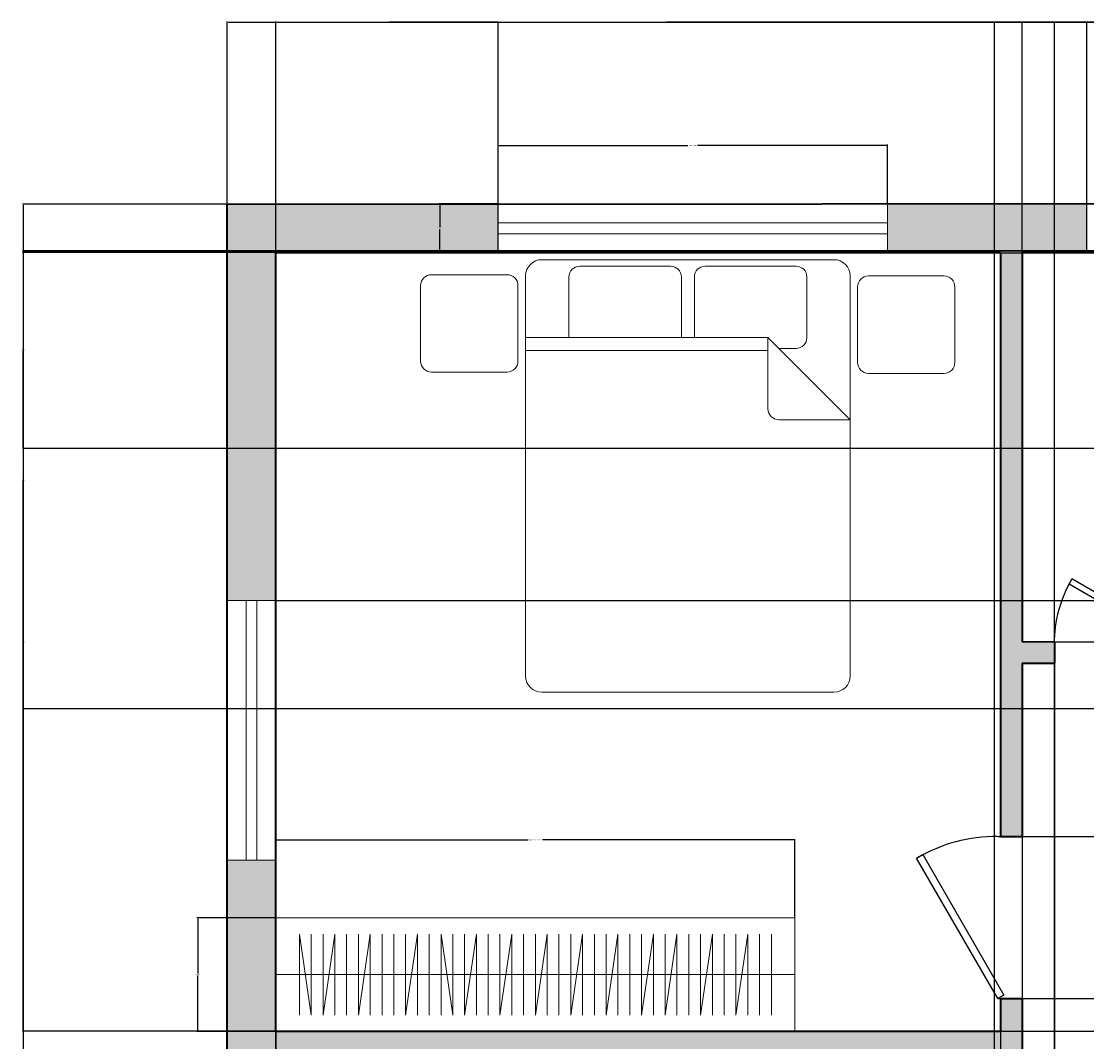
# Model space of a CAD drawing. Units: inches. Extents: x 1531 to 2263, y 2711 to 3216.
# Tile 4 of 12: x 1531 to 1728, y 3028 to 3216. Entities that reach past the tile are written whole.
import ezdxf

# ---------------------------------------------------------------- set-up
doc = ezdxf.new("R2010")
doc.units = ezdxf.units.IN
for name, color, linetype, lineweight in [('A-ANNO-DIMS', 2, 'Continuous', 18), ('A-DOOR', 3, 'Continuous', 25), ('A-FLOR-CASE', 9, 'Continuous', 18), ('A-FURN', 8, 'Continuous', 18), ('A-GLAZ', 4, 'Continuous', 18), ('A-WALL', 7, 'Continuous', 35)]:
    doc.layers.add(name, color=color, linetype=linetype, lineweight=lineweight)
doc.layers.add('A-WALL-PATT', color=18, linetype='Continuous', lineweight=13, true_color=0x000000)
doc.styles.get("Standard").update_dxf_attribs({"font": 'arial.ttf'})
doc.dimstyles.get("Standard").update_dxf_attribs({"dimtxt": 0.18, "dimasz": 0.18, "dimexe": 0.18, "dimexo": 0.0625, "dimgap": 0.09, "dimtad": 0, "dimtih": 1, "dimtoh": 1, "dimdec": 4, "dimzin": 0, "dimdsep": 46, "dimtxsty": 'Standard', "dimcen": 0.09, "dimadec": 0, "dimazin": 0, "dimtfac": 1, "dimtdec": 4, "dimtofl": 0, "dimtmove": 0, "dimatfit": 3, "dimfxl": 1, "dimtolj": 1, "dimtzin": 0, "dimarcsym": 0})

# ---------------------------------------------------------------- blocks, each defined once
blk = doc.blocks.new('*U3')
for p, q in [((0, 0), (0, -6)), ((40, 0), (40, -6))]:
    blk.add_line(p, q)
blk.add_lwpolyline([(0, 0), (34.64, 20), (35.52, 18.48), (0.87, -1.52)], close=True)
blk.add_arc((0, 0), 40, 0, 30)
blk = doc.blocks.new('*U4')
for p, q in [((-40, 0), (-40, 6)), ((0, 0), (0, 6))]:
    blk.add_line(p, q)
blk.add_lwpolyline([(0, 0), (-34.64, -20), (-35.52, -18.48), (-0.88, 1.52)], close=True)
blk.add_arc((0, 0), 40, 180, 210)
blk = doc.blocks.new('Bed - Queen')
for p, q in [((3, 0), (57, 0)), ((10, -1.2), (26.8, -1.2)), ((33.2, -1.2), (50, -1.2)), ((0, -77), (0, -3)), ((8, -14.4), (8, -3.2)), ((28.8, -3.2), (28.8, -14.4)), ((31.2, -14.4), (31.2, -3.2)), ((52, -3.2), (52, -14.4)), ((60, -3), (60, -77)), ((0, -14.4), (44.8, -14.4)), ((60, -29.6), (44.8, -14.4)), ((44.8, -14.4), (44.8, -27.6)), ((44.8, -16.8), (0, -16.8)), ((50, -16.4), (46.8, -16.4)), ((46.8, -29.6), (60, -29.6)), ((57, -80), (3, -80))]:
    blk.add_line(p, q)
blk.add_lwpolyline([(63.37, -3.02), (77.37, -3.02, -0.414214), (79.37, -5.02), (79.37, -19.02, -0.414214), (77.37, -21.02), (63.37, -21.02, -0.414214), (61.37, -19.02), (61.37, -5.02, -0.414214)], format="xyb", close=True)
for centre, radius, start, end in [((3, -3), 3, 90, 180), ((57, -3), 3, 0, 90), ((10, -3.2), 2, 90, 180), ((26.8, -3.2), 2, 0, 90), ((33.2, -3.2), 2, 90, 180), ((50, -3.2), 2, 0, 90), ((50, -14.4), 2, 270, 0), ((46.8, -27.6), 2, 180, 270), ((3, -77), 3, 180, 270), ((57, -77), 3, 270, 0)]:
    blk.add_arc(centre, radius, start, end)
blk = doc.blocks.new('WIN-72IN')
for p, q in [((0, 5.5), (72, 5.5)), ((0, 3.5), (72, 3.5))]:
    blk.add_line(p, q)
for points in [[(0, 9), (0, 0)], [(72, 0), (72, 9)]]:
    blk.add_lwpolyline(points)
blk = doc.blocks.new('WIN-48IN')
for p, q in [((3.5, 48), (3.5, 0)), ((5.5, 48), (5.5, 0))]:
    blk.add_line(p, q)
for points in [[(0, 48), (9, 48)], [(9, 0), (0, 0)]]:
    blk.add_lwpolyline(points)
blk = doc.blocks.new('WARDROBE-96IN')
for p, q in [((96, 21), (0, 21)), ((0, 21), (0, 0)), ((0, 0), (0, 21)), ((96, 0), (96, 21)), ((4.36, 3), (4.36, 18)), ((6.55, 3), (4.36, 18)), ((6.55, 3), (6.55, 18)), ((8.73, 3), (8.73, 18)), ((10.91, 18), (8.73, 3)), ((10.91, 3), (10.91, 18)), ((13.09, 3), (13.09, 18)), ((15.27, 3), (15.27, 18)), ((17.45, 18), (15.27, 3)), ((17.45, 3), (17.45, 18)), ((19.64, 3), (19.64, 18)), ((21.82, 3), (21.82, 18)), ((24, 3), (24, 18)), ((26.18, 18), (24, 3)), ((26.18, 3), (26.18, 18)), ((28.36, 3), (28.36, 18)), ((30.55, 3), (30.55, 18)), ((32.73, 3), (30.55, 18)), ((32.73, 3), (32.73, 18)), ((34.91, 3), (34.91, 18)), ((37.09, 18), (34.91, 3)), ((37.09, 3), (37.09, 18)), ((39.27, 3), (39.27, 18)), ((41.45, 3), (41.45, 18)), ((43.64, 18), (41.45, 3)), ((43.64, 3), (43.64, 18)), ((45.82, 3), (45.82, 18)), ((48, 3), (48, 18)), ((50.18, 18), (48, 3)), ((50.18, 3), (50.18, 18)), ((52.36, 3), (52.36, 18)), ((54.55, 3), (54.55, 18)), ((56.73, 18), (54.55, 3)), ((56.73, 3), (56.73, 18)), ((58.91, 3), (58.91, 18)), ((61.09, 3), (61.09, 18)), ((63.27, 18), (61.09, 3)), ((63.27, 3), (63.27, 18)), ((65.45, 3), (65.45, 18)), ((67.64, 3), (67.64, 18)), ((69.82, 18), (67.64, 3)), ((69.82, 3), (69.82, 18)), ((72, 3), (72, 18)), ((74.18, 18), (72, 3)), ((74.18, 3), (74.18, 18)), ((76.36, 3), (76.36, 18)), ((78.55, 3), (78.55, 18)), ((80.73, 18), (78.55, 3)), ((80.73, 3), (80.73, 18)), ((82.91, 3), (82.91, 18)), ((85.09, 3), (85.09, 18)), ((87.27, 18), (85.09, 3)), ((87.27, 3), (87.27, 18)), ((89.45, 3), (89.45, 18)), ((91.64, 3), (91.64, 18)), ((96, 10.5), (0, 10.5)), ((0, 0), (96, 0))]:
    blk.add_line(p, q)
blk = doc.blocks.new('*D26')
at = {"layer": 'A-ANNO-DIMS', "color": 0, "lineweight": -2, "transparency": 16777216}
for p, q in [((1619.02, 3182.76), (1619.02, 3193.68)), ((1691.02, 3182.76), (1691.02, 3193.68)), ((1619.2, 3193.5), (1654.13, 3193.5)), ((1690.84, 3193.5), (1655.92, 3193.5))]:
    blk.add_line(p, q, dxfattribs=at)
at = {"layer": 'A-ANNO-DIMS', "color": 0, "transparency": 16777216}
for points in [[(1619.2, 3193.53), (1619.2, 3193.47), (1619.02, 3193.5)], [(1690.84, 3193.53), (1690.84, 3193.47), (1691.02, 3193.5)]]:
    blk.add_solid(points, dxfattribs=at)
at = {"layer": 'Defpoints', "color": 0, "transparency": 16777216}
for p in [(1691.02, 3193.5), (1619.02, 3182.7), (1691.02, 3182.7)]:
    blk.add_point(p, dxfattribs=at)
at = {"layer": 'A-ANNO-DIMS', "color": 0, "transparency": 16777216, "insert": (1655.02, 3193.5), "char_height": 0.18, "attachment_point": 5}
blk.add_mtext('\\A1;WDW 72 TYP.', dxfattribs=at)
blk = doc.blocks.new('*D27')
at = {"layer": 'A-ANNO-DIMS', "color": 0, "lineweight": -2, "transparency": 16777216}
for p, q in [((1618.96, 3182.7), (1608.04, 3182.7)), ((1608.22, 3182.52), (1608.22, 3178.38)), ((1608.22, 3173.88), (1608.22, 3178.02)), ((1618.96, 3173.7), (1608.04, 3173.7))]:
    blk.add_line(p, q, dxfattribs=at)
at = {"layer": 'A-ANNO-DIMS', "color": 0, "transparency": 16777216}
for points in [[(1608.19, 3182.52), (1608.25, 3182.52), (1608.22, 3182.7)], [(1608.19, 3173.88), (1608.25, 3173.88), (1608.22, 3173.7)]]:
    blk.add_solid(points, dxfattribs=at)
at = {"layer": 'Defpoints', "color": 0, "transparency": 16777216}
for p in [(1608.22, 3182.7), (1619.02, 3182.7), (1619.02, 3173.7)]:
    blk.add_point(p, dxfattribs=at)
at = {"layer": 'A-ANNO-DIMS', "color": 0, "transparency": 16777216, "insert": (1608.22, 3178.2), "char_height": 0.18, "attachment_point": 5}
blk.add_mtext('\\A1;9 TYP.', dxfattribs=at)
blk = doc.blocks.new('*D34')
at = {"layer": 'A-ANNO-DIMS', "color": 0, "lineweight": -2, "transparency": 16777216}
for p, q in [((1577.91, 3050.74), (1577.91, 3065.26)), ((1578.09, 3065.08), (1624.6, 3065.08)), ((1673.73, 3065.08), (1627.22, 3065.08)), ((1673.91, 3050.74), (1673.91, 3065.26))]:
    blk.add_line(p, q, dxfattribs=at)
at = {"layer": 'A-ANNO-DIMS', "color": 0, "transparency": 16777216}
for points in [[(1578.09, 3065.11), (1578.09, 3065.05), (1577.91, 3065.08)], [(1673.73, 3065.11), (1673.73, 3065.05), (1673.91, 3065.08)]]:
    blk.add_solid(points, dxfattribs=at)
at = {"layer": 'Defpoints', "color": 0, "transparency": 16777216}
for p in [(1673.91, 3065.08), (1577.91, 3050.68), (1673.91, 3050.68)]:
    blk.add_point(p, dxfattribs=at)
at = {"layer": 'A-ANNO-DIMS', "color": 0, "transparency": 16777216, "insert": (1625.91, 3065.08), "char_height": 0.18, "attachment_point": 5}
blk.add_mtext('\\A1;WARDROBE 96 TYP.', dxfattribs=at)
blk = doc.blocks.new('*D35')
at = {"layer": 'A-ANNO-DIMS', "color": 0, "lineweight": -2, "transparency": 16777216}
for p, q in [((1577.85, 3050.68), (1563.33, 3050.68)), ((1563.51, 3050.5), (1563.51, 3040.36)), ((1563.51, 3029.86), (1563.51, 3040)), ((1577.85, 3029.68), (1563.33, 3029.68))]:
    blk.add_line(p, q, dxfattribs=at)
at = {"layer": 'A-ANNO-DIMS', "color": 0, "transparency": 16777216}
for points in [[(1563.48, 3050.5), (1563.54, 3050.5), (1563.51, 3050.68)], [(1563.48, 3029.86), (1563.54, 3029.86), (1563.51, 3029.68)]]:
    blk.add_solid(points, dxfattribs=at)
at = {"layer": 'Defpoints', "color": 0, "transparency": 16777216}
for p in [(1563.51, 3050.68), (1577.91, 3050.68), (1577.91, 3029.68)]:
    blk.add_point(p, dxfattribs=at)
at = {"layer": 'A-ANNO-DIMS', "color": 0, "transparency": 16777216, "insert": (1563.51, 3040.18), "char_height": 0.18, "attachment_point": 5}
blk.add_mtext('\\A1;21 TYP.', dxfattribs=at)
blk = doc.blocks.new('*D54')
at = {"layer": 'A-ANNO-DIMS', "color": 0, "lineweight": -2, "transparency": 16777216}
for p, q in [((1568.91, 3182.74), (1568.91, 3216.47)), ((1569.09, 3216.29), (1898.62, 3216.29)), ((2228.73, 3216.29), (1899.2, 3216.29)), ((2228.91, 3183.08), (2228.91, 3216.47))]:
    blk.add_line(p, q, dxfattribs=at)
at = {"layer": 'A-ANNO-DIMS', "color": 0, "transparency": 16777216}
for points in [[(1569.09, 3216.32), (1569.09, 3216.26), (1568.91, 3216.29)], [(2228.73, 3216.32), (2228.73, 3216.26), (2228.91, 3216.29)]]:
    blk.add_solid(points, dxfattribs=at)
at = {"layer": 'Defpoints', "color": 0, "transparency": 16777216}
for p in [(2228.91, 3216.29), (1568.91, 3182.67), (2228.91, 3183.02)]:
    blk.add_point(p, dxfattribs=at)
at = {"layer": 'A-ANNO-DIMS', "color": 0, "transparency": 16777216, "insert": (1898.91, 3216.29), "char_height": 0.18, "attachment_point": 5}
blk.add_mtext('\\A1;660', dxfattribs=at)
blk = doc.blocks.new('*D56')
at = {"layer": 'A-ANNO-DIMS', "color": 0, "lineweight": -2, "transparency": 16777216}
for p, q in [((1568.85, 3182.67), (1531.04, 3182.67)), ((1531.22, 3182.49), (1531.22, 2972.86)), ((1531.22, 2762.85), (1531.22, 2972.49)), ((1568.85, 2762.67), (1531.04, 2762.67))]:
    blk.add_line(p, q, dxfattribs=at)
at = {"layer": 'A-ANNO-DIMS', "color": 0, "transparency": 16777216}
for points in [[(1531.19, 3182.49), (1531.25, 3182.49), (1531.22, 3182.67)], [(1531.19, 2762.85), (1531.25, 2762.85), (1531.22, 2762.67)]]:
    blk.add_solid(points, dxfattribs=at)
at = {"layer": 'Defpoints', "color": 0, "transparency": 16777216}
for p in [(1568.91, 3182.67), (1531.22, 2762.67), (1568.91, 2762.67)]:
    blk.add_point(p, dxfattribs=at)
at = {"layer": 'A-ANNO-DIMS', "color": 0, "transparency": 16777216, "insert": (1531.22, 2972.67), "char_height": 0.18, "attachment_point": 5}
blk.add_mtext('\\A1;420', dxfattribs=at)
blk = doc.blocks.new('*D57')
at = {"layer": 'A-ANNO-DIMS', "color": 0, "lineweight": -2, "transparency": 16777216}
for p, q in [((1577.91, 3029.62), (1577.91, 2711.06)), ((1711.91, 3029.69), (1711.91, 2711.06)), ((1578.09, 2711.24), (1644.63, 2711.24)), ((1711.73, 2711.24), (1645.19, 2711.24))]:
    blk.add_line(p, q, dxfattribs=at)
at = {"layer": 'A-ANNO-DIMS', "color": 0, "transparency": 16777216}
for points in [[(1578.09, 2711.27), (1578.09, 2711.21), (1577.91, 2711.24)], [(1711.73, 2711.27), (1711.73, 2711.21), (1711.91, 2711.24)]]:
    blk.add_solid(points, dxfattribs=at)
at = {"layer": 'Defpoints', "color": 0, "transparency": 16777216}
for p in [(1577.91, 3029.68), (1711.91, 3029.75), (1711.91, 2711.24)]:
    blk.add_point(p, dxfattribs=at)
at = {"layer": 'A-ANNO-DIMS', "color": 0, "transparency": 16777216, "insert": (1644.91, 2711.24), "char_height": 0.18, "attachment_point": 5}
blk.add_mtext('\\A1;134', dxfattribs=at)
blk = doc.blocks.new('*D58')
at = {"layer": 'A-ANNO-DIMS', "color": 0, "lineweight": -2, "transparency": 16777216}
for p, q in [((1715.91, 3097.69), (1715.91, 2711.06)), ((1775.91, 3097.72), (1775.91, 2711.06)), ((1716.09, 2711.24), (1745.69, 2711.24)), ((1775.73, 2711.24), (1746.13, 2711.24))]:
    blk.add_line(p, q, dxfattribs=at)
at = {"layer": 'A-ANNO-DIMS', "color": 0, "transparency": 16777216}
for points in [[(1716.09, 2711.27), (1716.09, 2711.21), (1715.91, 2711.24)], [(1775.73, 2711.27), (1775.73, 2711.21), (1775.91, 2711.24)]]:
    blk.add_solid(points, dxfattribs=at)
at = {"layer": 'Defpoints', "color": 0, "transparency": 16777216}
for p in [(1715.91, 3097.75), (1775.91, 3097.78), (1775.91, 2711.24)]:
    blk.add_point(p, dxfattribs=at)
at = {"layer": 'A-ANNO-DIMS', "color": 0, "transparency": 16777216, "insert": (1745.91, 2711.24), "char_height": 0.18, "attachment_point": 5}
blk.add_mtext('\\A1;60', dxfattribs=at)
blk = doc.blocks.new('*D63')
at = {"layer": 'A-ANNO-DIMS', "color": 0, "lineweight": -2, "transparency": 16777216}
for p, q in [((1711.85, 3173.75), (1531.04, 3173.75)), ((1531.22, 3173.57), (1531.22, 3101.93)), ((1531.22, 3029.93), (1531.22, 3101.57)), ((1711.85, 3029.75), (1531.04, 3029.75))]:
    blk.add_line(p, q, dxfattribs=at)
at = {"layer": 'A-ANNO-DIMS', "color": 0, "transparency": 16777216}
for points in [[(1531.19, 3173.57), (1531.25, 3173.57), (1531.22, 3173.75)], [(1531.19, 3029.93), (1531.25, 3029.93), (1531.22, 3029.75)]]:
    blk.add_solid(points, dxfattribs=at)
at = {"layer": 'Defpoints', "color": 0, "transparency": 16777216}
for p in [(1711.91, 3173.75), (1531.22, 3029.75), (1711.91, 3029.75)]:
    blk.add_point(p, dxfattribs=at)
at = {"layer": 'A-ANNO-DIMS', "color": 0, "transparency": 16777216, "insert": (1531.22, 3101.75), "char_height": 0.18, "attachment_point": 5}
blk.add_mtext('\\A1;144', dxfattribs=at)
blk = doc.blocks.new('*D66')
at = {"layer": 'A-ANNO-DIMS', "color": 0, "lineweight": -2, "transparency": 16777216}
for p, q in [((1577.91, 2895.74), (1577.91, 3216.47)), ((1578.09, 3216.29), (1676.63, 3216.29)), ((1775.73, 3216.29), (1677.19, 3216.29)), ((1775.91, 2895.85), (1775.91, 3216.47))]:
    blk.add_line(p, q, dxfattribs=at)
at = {"layer": 'A-ANNO-DIMS', "color": 0, "transparency": 16777216}
for points in [[(1578.09, 3216.32), (1578.09, 3216.26), (1577.91, 3216.29)], [(1775.73, 3216.32), (1775.73, 3216.26), (1775.91, 3216.29)]]:
    blk.add_solid(points, dxfattribs=at)
at = {"layer": 'Defpoints', "color": 0, "transparency": 16777216}
for p in [(1775.91, 3216.29), (1577.91, 2895.68), (1775.91, 2895.78)]:
    blk.add_point(p, dxfattribs=at)
at = {"layer": 'A-ANNO-DIMS', "color": 0, "transparency": 16777216, "insert": (1676.91, 3216.29), "char_height": 0.18, "attachment_point": 5}
blk.add_mtext('\\A1;198', dxfattribs=at)
blk = doc.blocks.new('*D80')
at = {"layer": 'A-ANNO-DIMS', "color": 0, "lineweight": -2, "transparency": 16777216}
for p, q in [((1715.97, 3173.75), (2262.37, 3173.75)), ((2262.19, 3173.57), (2262.19, 3137.93)), ((2262.19, 3101.93), (2262.19, 3137.57)), ((1715.97, 3101.75), (2262.37, 3101.75))]:
    blk.add_line(p, q, dxfattribs=at)
at = {"layer": 'A-ANNO-DIMS', "color": 0, "transparency": 16777216}
for points in [[(2262.16, 3173.57), (2262.22, 3173.57), (2262.19, 3173.75)], [(2262.16, 3101.93), (2262.22, 3101.93), (2262.19, 3101.75)]]:
    blk.add_solid(points, dxfattribs=at)
at = {"layer": 'Defpoints', "color": 0, "transparency": 16777216}
for p in [(1715.91, 3173.75), (1715.91, 3101.75), (2262.19, 3101.75)]:
    blk.add_point(p, dxfattribs=at)
at = {"layer": 'A-ANNO-DIMS', "color": 0, "transparency": 16777216, "insert": (2262.19, 3137.75), "char_height": 0.18, "attachment_point": 5}
blk.add_mtext('\\A1;72', dxfattribs=at)
blk = doc.blocks.new('*D85')
at = {"layer": 'A-ANNO-DIMS', "color": 0, "lineweight": -2, "transparency": 16777216}
for p, q in [((2079.85, 3173.94), (1531.04, 3173.94)), ((1531.22, 3173.76), (1531.22, 3131.82)), ((1531.22, 3089.52), (1531.22, 3131.46)), ((2079.85, 3089.34), (1531.04, 3089.34))]:
    blk.add_line(p, q, dxfattribs=at)
at = {"layer": 'A-ANNO-DIMS', "color": 0, "transparency": 16777216}
for points in [[(1531.19, 3173.76), (1531.25, 3173.76), (1531.22, 3173.94)], [(1531.19, 3089.52), (1531.25, 3089.52), (1531.22, 3089.34)]]:
    blk.add_solid(points, dxfattribs=at)
at = {"layer": 'Defpoints', "color": 0, "transparency": 16777216}
for p in [(1531.22, 3173.94), (2079.91, 3173.94), (2079.91, 3089.34)]:
    blk.add_point(p, dxfattribs=at)
at = {"layer": 'A-ANNO-DIMS', "color": 0, "transparency": 16777216, "insert": (1531.22, 3131.64), "char_height": 0.18, "attachment_point": 5}
blk.add_mtext('\\A1;84.6', dxfattribs=at)
blk = doc.blocks.new('*D86')
at = {"layer": 'A-ANNO-DIMS', "color": 0, "lineweight": -2, "transparency": 16777216}
for p, q in [((1715.97, 3065.75), (2262.37, 3065.75)), ((2262.19, 3065.57), (2262.19, 3050.93)), ((2262.19, 3035.93), (2262.19, 3050.57)), ((1715.97, 3035.75), (2262.37, 3035.75))]:
    blk.add_line(p, q, dxfattribs=at)
at = {"layer": 'A-ANNO-DIMS', "color": 0, "transparency": 16777216}
for points in [[(2262.16, 3065.57), (2262.22, 3065.57), (2262.19, 3065.75)], [(2262.16, 3035.93), (2262.22, 3035.93), (2262.19, 3035.75)]]:
    blk.add_solid(points, dxfattribs=at)
at = {"layer": 'Defpoints', "color": 0, "transparency": 16777216}
for p in [(1715.91, 3065.75), (2262.19, 3065.75), (1715.91, 3035.75)]:
    blk.add_point(p, dxfattribs=at)
at = {"layer": 'A-ANNO-DIMS', "color": 0, "transparency": 16777216, "insert": (2262.19, 3050.75), "char_height": 0.18, "attachment_point": 5}
blk.add_mtext('\\A1;30', dxfattribs=at)
blk = doc.blocks.new('*D87')
at = {"layer": 'A-ANNO-DIMS', "color": 0, "lineweight": -2, "transparency": 16777216}
for p, q in [((1721.91, 3101.69), (1721.91, 2711.06)), ((1745.91, 3101.7), (1745.91, 2711.06)), ((1722.09, 2711.24), (1733.69, 2711.24)), ((1745.73, 2711.24), (1734.13, 2711.24))]:
    blk.add_line(p, q, dxfattribs=at)
at = {"layer": 'A-ANNO-DIMS', "color": 0, "transparency": 16777216}
for points in [[(1722.09, 2711.27), (1722.09, 2711.21), (1721.91, 2711.24)], [(1745.73, 2711.27), (1745.73, 2711.21), (1745.91, 2711.24)]]:
    blk.add_solid(points, dxfattribs=at)
at = {"layer": 'Defpoints', "color": 0, "transparency": 16777216}
for p in [(1721.91, 3101.75), (1745.91, 3101.77), (1745.91, 2711.24)]:
    blk.add_point(p, dxfattribs=at)
at = {"layer": 'A-ANNO-DIMS', "color": 0, "transparency": 16777216, "insert": (1733.91, 2711.24), "char_height": 0.18, "attachment_point": 5}
blk.add_mtext('\\A1;24', dxfattribs=at)
blk = doc.blocks.new('*D88')
at = {"layer": 'A-ANNO-DIMS', "color": 0, "lineweight": -2, "transparency": 16777216}
for p, q in [((1577.91, 3173.74), (1577.91, 3216.47)), ((1578.09, 3216.29), (1598.09, 3216.29)), ((1618.84, 3216.29), (1598.85, 3216.29)), ((1619.02, 3173.76), (1619.02, 3216.47))]:
    blk.add_line(p, q, dxfattribs=at)
at = {"layer": 'A-ANNO-DIMS', "color": 0, "transparency": 16777216}
for points in [[(1578.09, 3216.32), (1578.09, 3216.26), (1577.91, 3216.29)], [(1618.84, 3216.32), (1618.84, 3216.26), (1619.02, 3216.29)]]:
    blk.add_solid(points, dxfattribs=at)
at = {"layer": 'Defpoints', "color": 0, "transparency": 16777216}
for p in [(1619.02, 3216.29), (1577.91, 3173.68), (1619.02, 3173.7)]:
    blk.add_point(p, dxfattribs=at)
at = {"layer": 'A-ANNO-DIMS', "color": 0, "transparency": 16777216, "insert": (1598.47, 3216.29), "char_height": 0.18, "attachment_point": 5}
blk.add_mtext('\\A1;41.11', dxfattribs=at)
blk = doc.blocks.new('*D89')
at = {"layer": 'A-ANNO-DIMS', "color": 0, "lineweight": -2, "transparency": 16777216}
for p, q in [((1715.91, 3173.81), (1715.91, 3216.47)), ((1716.09, 3216.29), (1721.43, 3216.29)), ((1727.68, 3216.29), (1722.34, 3216.29)), ((1727.86, 3173.82), (1727.86, 3216.47))]:
    blk.add_line(p, q, dxfattribs=at)
at = {"layer": 'A-ANNO-DIMS', "color": 0, "transparency": 16777216}
for points in [[(1716.09, 3216.32), (1716.09, 3216.26), (1715.91, 3216.29)], [(1727.68, 3216.32), (1727.68, 3216.26), (1727.86, 3216.29)]]:
    blk.add_solid(points, dxfattribs=at)
at = {"layer": 'Defpoints', "color": 0, "transparency": 16777216}
for p in [(1727.86, 3216.29), (1715.91, 3173.75), (1727.86, 3173.76)]:
    blk.add_point(p, dxfattribs=at)
at = {"layer": 'A-ANNO-DIMS', "color": 0, "transparency": 16777216, "insert": (1721.89, 3216.29), "char_height": 0.18, "attachment_point": 5}
blk.add_mtext('\\A1;11.954', dxfattribs=at)
blk = doc.blocks.new('*D100')
at = {"layer": 'A-ANNO-DIMS', "color": 0, "lineweight": -2, "transparency": 16777216}
for p, q in [((2219.85, 3174.02), (1531.04, 3174.02)), ((1531.22, 3173.84), (1531.22, 3155.93)), ((1531.22, 3137.67), (1531.22, 3155.57)), ((2219.85, 3137.49), (1531.04, 3137.49))]:
    blk.add_line(p, q, dxfattribs=at)
at = {"layer": 'A-ANNO-DIMS', "color": 0, "transparency": 16777216}
for points in [[(1531.19, 3173.84), (1531.25, 3173.84), (1531.22, 3174.02)], [(1531.19, 3137.67), (1531.25, 3137.67), (1531.22, 3137.49)]]:
    blk.add_solid(points, dxfattribs=at)
at = {"layer": 'Defpoints', "color": 0, "transparency": 16777216}
for p in [(2219.91, 3174.02), (1531.22, 3137.49), (2219.91, 3137.49)]:
    blk.add_point(p, dxfattribs=at)
at = {"layer": 'A-ANNO-DIMS', "color": 0, "transparency": 16777216, "insert": (1531.22, 3155.75), "char_height": 0.18, "attachment_point": 5}
blk.add_mtext('\\A1;36.526', dxfattribs=at)
blk = doc.blocks.new('*D103')
at = {"layer": 'A-ANNO-DIMS', "color": 0, "lineweight": -2, "transparency": 16777216}
for p, q in [((1577.97, 3173.68), (2262.37, 3173.68)), ((2262.19, 3173.5), (2262.19, 3141.71)), ((2262.19, 3109.55), (2262.19, 3141.34)), ((1577.97, 3109.37), (2262.37, 3109.37))]:
    blk.add_line(p, q, dxfattribs=at)
at = {"layer": 'A-ANNO-DIMS', "color": 0, "transparency": 16777216}
for points in [[(2262.16, 3173.5), (2262.22, 3173.5), (2262.19, 3173.68)], [(2262.16, 3109.55), (2262.22, 3109.55), (2262.19, 3109.37)]]:
    blk.add_solid(points, dxfattribs=at)
at = {"layer": 'Defpoints', "color": 0, "transparency": 16777216}
for p in [(1577.91, 3173.68), (1577.91, 3109.37), (2262.19, 3109.37)]:
    blk.add_point(p, dxfattribs=at)
at = {"layer": 'A-ANNO-DIMS', "color": 0, "transparency": 16777216, "insert": (2262.19, 3141.52), "char_height": 0.18, "attachment_point": 5}
blk.add_mtext('\\A1;64.31', dxfattribs=at)
blk = doc.blocks.new('*D110')
at = {"layer": 'A-ANNO-DIMS', "color": 0, "lineweight": -2, "transparency": 16777216}
for p, q in [((1711.97, 3035.75), (2262.37, 3035.75)), ((2262.19, 3035.57), (2262.19, 3032.93)), ((2262.19, 3029.93), (2262.19, 3032.57)), ((1711.97, 3029.75), (2262.37, 3029.75))]:
    blk.add_line(p, q, dxfattribs=at)
at = {"layer": 'A-ANNO-DIMS', "color": 0, "transparency": 16777216}
for points in [[(2262.16, 3035.57), (2262.22, 3035.57), (2262.19, 3035.75)], [(2262.16, 3029.93), (2262.22, 3029.93), (2262.19, 3029.75)]]:
    blk.add_solid(points, dxfattribs=at)
at = {"layer": 'Defpoints', "color": 0, "transparency": 16777216}
for p in [(1711.91, 3035.75), (2262.19, 3035.75), (1711.91, 3029.75)]:
    blk.add_point(p, dxfattribs=at)
at = {"layer": 'A-ANNO-DIMS', "color": 0, "transparency": 16777216, "insert": (2262.19, 3032.75), "char_height": 0.18, "attachment_point": 5}
blk.add_mtext('\\A1;6', dxfattribs=at)
blk = doc.blocks.new('*D111')
at = {"layer": 'A-ANNO-DIMS', "color": 0, "lineweight": -2, "transparency": 16777216}
for p, q in [((1577.91, 3010), (1577.91, 3216.47)), ((1578.09, 3216.29), (1649.63, 3216.29)), ((1721.73, 3216.29), (1650.19, 3216.29)), ((1721.91, 3010), (1721.91, 3216.47))]:
    blk.add_line(p, q, dxfattribs=at)
at = {"layer": 'A-ANNO-DIMS', "color": 0, "transparency": 16777216}
for points in [[(1578.09, 3216.32), (1578.09, 3216.26), (1577.91, 3216.29)], [(1721.73, 3216.32), (1721.73, 3216.26), (1721.91, 3216.29)]]:
    blk.add_solid(points, dxfattribs=at)
at = {"layer": 'Defpoints', "color": 0, "transparency": 16777216}
for p in [(1721.91, 3216.29), (1577.91, 3009.94), (1721.91, 3009.94)]:
    blk.add_point(p, dxfattribs=at)
at = {"layer": 'A-ANNO-DIMS', "color": 0, "transparency": 16777216, "insert": (1649.91, 3216.29), "char_height": 0.18, "attachment_point": 5}
blk.add_mtext('\\A1;144', dxfattribs=at)
blk = doc.blocks.new('*D128')
at = {"layer": 'A-ANNO-DIMS', "color": 0, "lineweight": -2, "transparency": 16777216}
for p, q in [((1710.84, 2841.9), (1710.84, 3216.47)), ((1711.02, 3216.29), (1721.3, 3216.29)), ((1732.52, 3216.29), (1722.23, 3216.29)), ((1732.7, 2841.9), (1732.7, 3216.47))]:
    blk.add_line(p, q, dxfattribs=at)
at = {"layer": 'A-ANNO-DIMS', "color": 0, "transparency": 16777216}
for points in [[(1711.02, 3216.32), (1711.02, 3216.26), (1710.84, 3216.29)], [(1732.52, 3216.32), (1732.52, 3216.26), (1732.7, 3216.29)]]:
    blk.add_solid(points, dxfattribs=at)
at = {"layer": 'Defpoints', "color": 0, "transparency": 16777216}
for p in [(1732.7, 3216.29), (1710.84, 2841.84), (1732.7, 2841.84)]:
    blk.add_point(p, dxfattribs=at)
at = {"layer": 'A-ANNO-DIMS', "color": 0, "transparency": 16777216, "insert": (1721.77, 3216.29), "char_height": 0.18, "attachment_point": 5}
blk.add_mtext('\\A1;21.866', dxfattribs=at)

msp = doc.modelspace()

# ---------------------------------------------------------------- hatches: boundary and pattern name
at = {"layer": 'A-WALL-PATT'}
h = msp.add_hatch(color=256, dxfattribs=at)
h.dxf.hatch_style = 1
h.paths.add_polyline_path([(1577.9111, 3173.6796), (1619.0249, 3173.7011), (1619.0249, 3182.7011), (1568.9111, 3182.6749), (1568.9111, 3109.3695), (1577.9111, 3109.3695)])
h = msp.add_hatch(color=256, dxfattribs=at)
h.dxf.hatch_style = 1
h.paths.add_polyline_path([(1727.8638, 3182.758), (1691.0249, 3182.7387), (1691.0249, 3173.7387), (1711.9101, 3173.7496), (1711.9101, 3065.7517), (1715.9101, 3065.7517), (1715.9101, 3097.7517), (1721.9101, 3097.7549), (1721.9101, 3101.3517), (1721.9101, 3101.7549), (1715.9101, 3101.7517), (1715.9101, 3173.7517), (1727.8638, 3173.758)])
h = msp.add_hatch(color=256, dxfattribs=at)
h.dxf.hatch_style = 1
h.paths.add_polyline_path([(1715.9101, 3035.7517), (1711.9101, 3035.7496), (1711.9101, 3029.7496), (1673.9111, 3029.7297), (1673.9111, 3029.6795), (1577.9111, 3029.6795), (1577.9111, 3050.6795), (1577.9111, 3061.3695), (1568.9111, 3061.3695), (1568.9111, 3025.6795), (1577.9111, 3025.6795), (1715.9101, 3025.7517)])

# ---------------------------------------------------------------- linework, layer by layer
at = {"layer": 'A-FURN'}
msp.add_lwpolyline([(1620.6798, 3169.612), (1606.6798, 3169.612, 0.41421356), (1604.6798, 3167.612), (1604.6798, 3153.612, 0.41421356), (1606.6798, 3151.612), (1620.6798, 3151.612, 0.41421356), (1622.6798, 3153.612), (1622.6798, 3167.612, 0.41421356)], format="xyb", close=True, dxfattribs=at)
at = {"layer": 'A-WALL'}
for p, q in [((1577.9111, 3173.6796), (1711.9101, 3173.7496)), ((1577.9111, 3029.6795), (1577.9111, 3173.6796)), ((1711.9101, 3173.7496), (1711.9101, 3065.7496)), ((1715.9101, 3173.7517), (1775.9101, 3173.7831)), ((1715.9101, 3173.7517), (1715.9101, 3101.7517)), ((1715.9101, 3101.7517), (1721.9101, 3101.7549)), ((1721.9101, 3101.7549), (1721.9101, 3097.7517)), ((1715.9101, 3097.7517), (1721.9101, 3097.7549)), ((1715.9101, 3097.7517), (1715.9101, 3065.7517)), ((1711.9101, 3065.7496), (1715.9101, 3065.7517)), ((1711.907, 3035.7496), (1715.9101, 3035.7517)), ((1711.9101, 3035.7496), (1711.9101, 3029.7496)), ((1715.9101, 3035.7517), (1715.9101, 3025.7517)), ((1577.9111, 3029.6795), (1711.9101, 3029.7496))]:
    msp.add_line(p, q, dxfattribs=at)
msp.add_lwpolyline([(1933.9101, 2762.8657), (1568.9111, 2762.6748), (1568.9111, 3182.6749), (2228.9101, 3183.02), (2228.9101, 2798.8631)], dxfattribs=at)

# ---------------------------------------------------------------- block references
at = {"layer": 'A-DOOR', "xscale": -0.6, "yscale": 0.6, "zscale": 0.6}
msp.add_blockref('*U3', (1745.9101, 3101.3517), dxfattribs=at)
at = {"layer": 'A-DOOR', "xscale": 0.75, "yscale": 0.75, "zscale": 0.75, "rotation": 270}
msp.add_blockref('*U4', (1711.4101, 3035.7517), dxfattribs=at)
at = {"layer": 'A-FLOR-CASE'}
msp.add_blockref('WARDROBE-96IN', (1577.911, 3029.68), dxfattribs=at)
at = {"layer": 'A-FURN'}
msp.add_blockref('Bed - Queen', (1624.1141, 3172.3959), dxfattribs=at)
at = {"layer": 'A-GLAZ'}
for name, p in [('WIN-72IN', (1619.025, 3173.701)), ('WIN-48IN', (1568.911, 3061.37))]:
    msp.add_blockref(name, p, dxfattribs=at)

# ---------------------------------------------------------------- dimensions: what is measured, and where the dimension line sits
at = {"layer": 'A-ANNO-DIMS'}
for base, p1, p2, override, picture, middle in [((2228.9101, 3216.295), (1568.9111, 3182.6749), (2228.9101, 3183.02), {"dimdec": 0, "dimlfac": 1, "dimrnd": 0, "dimzin": 0, "dimdsep": 46, "dimlunit": 2}, '*D54', (1898.9106, 3216.295)), ((1775.9101, 3216.295), (1577.9111, 2895.6796), (1775.9101, 2895.7831), {"dimdec": 0, "dimlfac": 1, "dimrnd": 0, "dimzin": 0, "dimdsep": 46, "dimlunit": 2}, '*D66', (1676.9106, 3216.295)), ((1619.0249, 3216.295), (1577.9111, 3173.6796), (1619.0249, 3173.7011), {"dimdec": 2, "dimlfac": 1, "dimrnd": 0, "dimzin": 0, "dimdsep": 46, "dimlunit": 2}, '*D88', (1598.468, 3216.295)), ((1721.9111, 3216.295), (1577.9111, 3009.9378), (1721.9111, 3009.9378), {"dimdec": 0, "dimlfac": 1, "dimrnd": 0, "dimzin": 0, "dimdsep": 46, "dimlunit": 2}, '*D111', (1649.9111, 3216.295)), ((1732.7021, 3216.295), (1710.8363, 2841.8359), (1732.7021, 2841.8359), {"dimdec": 3, "dimlfac": 1, "dimrnd": 0, "dimzin": 0, "dimdsep": 46, "dimlunit": 2}, '*D128', (1721.7692, 3216.295)), ((1727.8638, 3216.295), (1715.9101, 3173.7517), (1727.8638, 3173.758), {"dimdec": 3, "dimlfac": 1, "dimrnd": 0, "dimzin": 0, "dimdsep": 46, "dimlunit": 2}, '*D89', (1721.887, 3216.295)), ((1745.9101, 2711.2407), (1721.9101, 3101.7549), (1745.9101, 3101.7674), {"dimdec": 0, "dimlfac": 1, "dimrnd": 0, "dimzin": 0, "dimdsep": 46, "dimlunit": 2}, '*D87', (1733.9101, 2711.2407)), ((1775.9101, 2711.2407), (1715.9101, 3097.7517), (1775.9101, 3097.7831), {"dimdec": 0, "dimlfac": 1, "dimrnd": 0, "dimzin": 0, "dimdsep": 46, "dimlunit": 2}, '*D58', (1745.9101, 2711.2407)), ((1711.9101, 2711.2407), (1577.9111, 3029.6795), (1711.9101, 3029.7496), {"dimdec": 0, "dimlfac": 1, "dimrnd": 0, "dimzin": 0, "dimdsep": 46, "dimlunit": 2}, '*D57', (1644.9106, 2711.2407))]:
    dim = msp.add_linear_dim(base=base, p1=p1, p2=p2, dimstyle='Standard', override=override, dxfattribs=at)
    dim.commit()
    dim.dimension.update_dxf_attribs({"geometry": picture, "text_midpoint": middle})
for base, p1, p2, text, picture, middle in [((1691.0249, 3193.5011), (1619.0249, 3182.7011), (1691.0249, 3182.7011), 'WDW <> TYP.', '*D26', (1655.0249, 3193.5011)), ((1673.9111, 3065.0795), (1577.9111, 3050.6795), (1673.9111, 3050.6795), 'WARDROBE <> TYP.', '*D34', (1625.9111, 3065.0795))]:
    dim = msp.add_linear_dim(base=base, p1=p1, p2=p2, text=text, dimstyle='Standard', override={"dimdec": 0, "dimlfac": 1, "dimrnd": 0, "dimzin": 0, "dimdsep": 46, "dimlunit": 2}, dxfattribs=at)
    dim.commit()
    dim.dimension.update_dxf_attribs({"geometry": picture, "text_midpoint": middle})
for base, p1, p2, override, picture, middle in [((1531.2212, 2762.6748), (1568.9111, 3182.6749), (1568.9111, 2762.6748), {"dimdec": 0, "dimlfac": 1, "dimrnd": 0, "dimzin": 0, "dimdsep": 46, "dimlunit": 2}, '*D56', (1531.2212, 2972.6748)), ((1531.2212, 3137.4897), (2219.9101, 3174.0153), (2219.9101, 3137.4897), {"dimdec": 3, "dimlfac": 1, "dimrnd": 0, "dimzin": 0, "dimdsep": 46, "dimlunit": 2}, '*D100', (1531.2212, 3155.7525)), ((1531.2212, 3173.9421), (2079.9101, 3089.343), (2079.9101, 3173.9421), {"dimdec": 1, "dimlfac": 1, "dimrnd": 0, "dimzin": 0, "dimdsep": 46, "dimlunit": 2}, '*D85', (1531.2212, 3131.6425)), ((1531.2212, 3029.7496), (1711.9101, 3173.7496), (1711.9101, 3029.7496), {"dimdec": 0, "dimlfac": 1, "dimrnd": 0, "dimzin": 0, "dimdsep": 46, "dimlunit": 2}, '*D63', (1531.2212, 3101.7496)), ((2262.1851, 3109.3695), (1577.9111, 3173.6796), (1577.9111, 3109.3695), {"dimdec": 2, "dimlfac": 1, "dimrnd": 0, "dimzin": 0, "dimdsep": 46, "dimlunit": 2}, '*D103', (2262.1851, 3141.5245)), ((2262.1851, 3101.7517), (1715.9101, 3173.7517), (1715.9101, 3101.7517), {"dimdec": 0, "dimlfac": 1, "dimrnd": 0, "dimzin": 0, "dimdsep": 46, "dimlunit": 2}, '*D80', (2262.1851, 3137.7517)), ((2262.1851, 3065.7517), (1715.9101, 3035.7517), (1715.9101, 3065.7517), {"dimdec": 0, "dimlfac": 1, "dimrnd": 0, "dimzin": 0, "dimdsep": 46, "dimlunit": 2}, '*D86', (2262.1851, 3050.7517)), ((2262.1851, 3035.7496), (1711.9101, 3029.7496), (1711.9101, 3035.7496), {"dimdec": 0, "dimlfac": 1, "dimrnd": 0, "dimzin": 0, "dimdsep": 46, "dimlunit": 2}, '*D110', (2262.1851, 3032.7496))]:
    dim = msp.add_linear_dim(base=base, p1=p1, p2=p2, angle=90, dimstyle='Standard', override=override, dxfattribs=at)
    dim.commit()
    dim.dimension.update_dxf_attribs({"geometry": picture, "text_midpoint": middle})
for base, p1, p2, picture, middle in [((1608.2249, 3182.7011), (1619.0249, 3173.7011), (1619.0249, 3182.7011), '*D27', (1608.2249, 3178.2011)), ((1563.5111, 3050.6795), (1577.9111, 3029.6795), (1577.9111, 3050.6795), '*D35', (1563.5111, 3040.1795))]:
    dim = msp.add_linear_dim(base=base, p1=p1, p2=p2, angle=90, text='<> TYP.', dimstyle='Standard', override={"dimdec": 0, "dimlfac": 1, "dimrnd": 0, "dimzin": 0, "dimdsep": 46, "dimlunit": 2}, dxfattribs=at)
    dim.commit()
    dim.dimension.update_dxf_attribs({"geometry": picture, "text_midpoint": middle})

doc.saveas('drawing.dxf')
